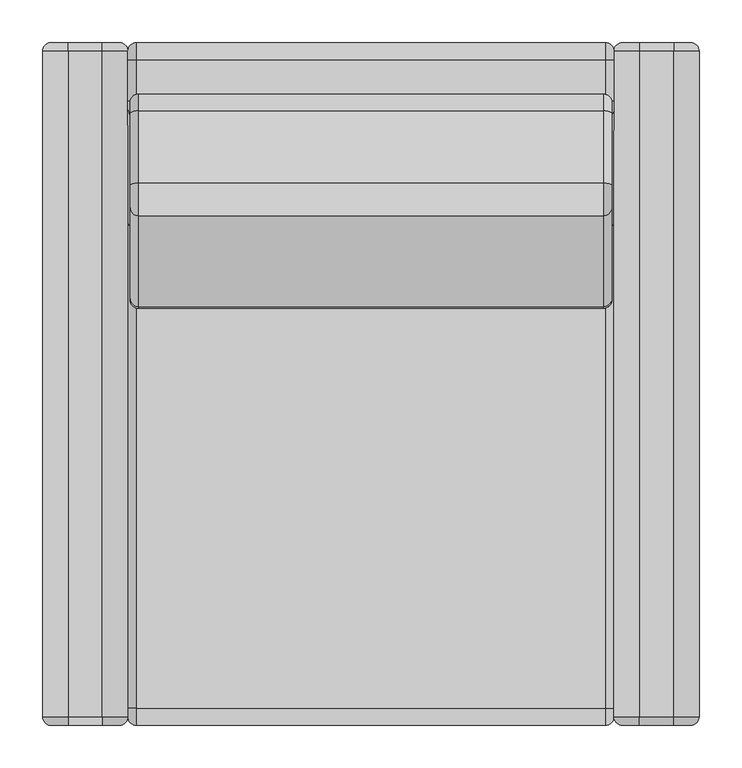
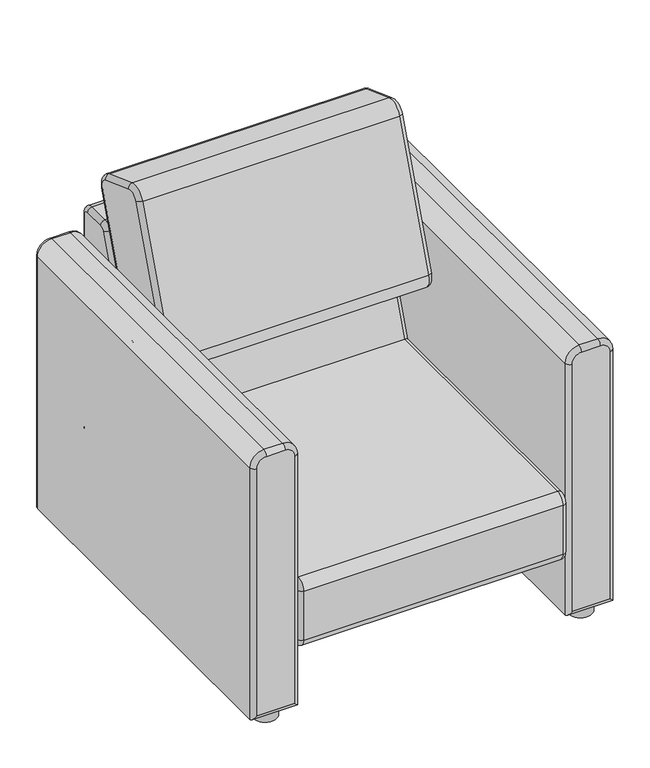
"""IFC4 building model written with IfcOpenShell, lengths in millimetres: furniture geometry."""

from ifc_helpers import new_model, si_unit, point, frame, frame_2d, origin, origin_with_axes, place, context, project, spatial, circle_curve, ellipse_curve, trimmed, segment, composite_curve, outline, extrude, source, transform, mapped, element, save
from ifc_brep_helpers import plane_surface, cylinder_surface, revolved_surface, advanced_brep


def furniture_f28dd14e(model_context):
    return source(origin(), model_context, "Body", "SolidModel", [
        advanced_brep(
        [(-375.0, 0.0, 590.0), (-375.0, 0.0, 35.0), (-295.0, 0.0, 35.0), (-295.0, 0.0, 590.0), (-315.0, 0.0, 610.0), (-355.0, 0.0, 610.0), (-295.0, 800.0, 590.0), (-295.0, 800.0, 35.0), (-375.0, 800.0, 35.0), (-375.0, 800.0, 590.0), (-355.0, 800.0, 610.0), (-315.0, 800.0, 610.0), (-285.0, 9.9999877, 590.0), (-285.0, 790.0000093, 590.0), (-315.0, 790.0, 620.0), (-315.0, 10.0, 620.0), (-355.0, 9.9999878, 620.0), (-355.0, 790.0, 620.0), (-385.0, 790.0, 590.0), (-385.0, 9.9999878, 590.0), (-285.0, 10.0, 25.0), (-285.0, 790.0, 25.0), (-385.0, 10.0, 25.0), (-385.0, 790.0, 25.0)],
        [
            (0, 1),
            (1, 2),
            (2, 3),
            (3, 4, circle_curve(frame((-315.0, 0.0, 590.0), z_axis=(0.0, -1.0, 0.0), x_axis=(0.0, 0.0, 1.0)), 20.0)),
            (4, 5),
            (5, 0, circle_curve(frame((-355.0, 0.0, 590.0), z_axis=(0.0, -1.0, 0.0), x_axis=(-1.0, 0.0, 0.0)), 20.0)),
            (6, 7),
            (7, 8),
            (8, 9),
            (9, 10, circle_curve(frame((-355.0, 800.0, 590.0), z_axis=(0.0, 1.0, 0.0), x_axis=(0.0, 0.0, 1.0)), 20.0)),
            (10, 11),
            (11, 6, circle_curve(frame((-315.0, 800.0, 590.0), z_axis=(0.0, 1.0, 0.0), x_axis=(1.0, 0.0, 0.0)), 20.0)),
            (12, 13),
            (13, 14, circle_curve(frame((-315.0, 790.0, 590.0), z_axis=(0.0, -1.0, 0.0), x_axis=(-1.0, 0.0, 0.0)), 30.0)),
            (14, 15),
            (15, 12, circle_curve(frame((-315.0, 10.0, 590.0), z_axis=(0.0, 1.0, 0.0), x_axis=(-1.0, 0.0, 0.0)), 30.0)),
            (16, 17),
            (17, 18, circle_curve(frame((-355.0, 790.0, 590.0), z_axis=(0.0, -1.0, 0.0), x_axis=(-1.0, 0.0, 0.0)), 30.0)),
            (18, 19),
            (19, 16, circle_curve(frame((-355.0, 10.0, 590.0), z_axis=(0.0, 1.0, 0.0), x_axis=(-1.0, 0.0, 0.0)), 30.0)),
            (20, 21),
            (21, 13),
            (12, 20),
            (22, 23),
            (23, 21),
            (20, 22),
            (18, 23),
            (22, 19),
            (14, 17),
            (16, 15),
            (19, 0, circle_curve(frame((-375.0, 10.0, 590.0), z_axis=(0.0, 0.0, 1.0), x_axis=(-1.0, 0.0, 0.0)), 10.0)),
            (5, 16, circle_curve(frame((-355.0, 10.0, 610.0), z_axis=(-1.0, 0.0, 0.0), x_axis=(0.0, 0.0, 1.0)), 10.0)),
            (4, 15, circle_curve(frame((-315.0, 10.0, 610.0), z_axis=(-1.0, 0.0, 0.0), x_axis=(0.0, 0.0, 1.0)), 10.0)),
            (3, 12, circle_curve(frame((-295.0, 10.0, 590.0), z_axis=(0.0, 0.0, 1.0), x_axis=(1.0, 0.0, 0.0)), 10.0)),
            (2, 20, ellipse_curve(frame((-295.0, 10.0, 35.0), z_axis=(0.7071067811865458, 0.0, 0.7071067811865492), x_axis=(0.7071067811865492, 0.0, -0.7071067811865458)), 14.1421356, 10.0)),
            (1, 22, ellipse_curve(frame((-375.0, 10.0, 35.0), z_axis=(0.7071067811865492, 0.0, -0.7071067811865457), x_axis=(-0.707106781186546, 0.0, -0.7071067811865491)), 14.1421356, 10.0)),
            (13, 6, circle_curve(frame((-295.0, 790.0, 590.0), z_axis=(0.0, 0.0, 1.0), x_axis=(-1.0, 0.0, 0.0)), 10.0)),
            (11, 14, circle_curve(frame((-315.0, 790.0, 610.0), z_axis=(1.0, 0.0, 0.0), x_axis=(0.0, 0.0, -1.0)), 10.0)),
            (10, 17, circle_curve(frame((-355.0, 790.0, 610.0), z_axis=(1.0, 0.0, 0.0), x_axis=(0.0, 0.0, -1.0)), 10.0)),
            (9, 18, circle_curve(frame((-375.0, 790.0, 590.0), z_axis=(0.0, 0.0, 1.0), x_axis=(1.0, 0.0, 0.0)), 10.0)),
            (8, 23, ellipse_curve(frame((-375.0, 790.0, 35.0), z_axis=(-0.7071067811865492, 0.0, 0.7071067811865458), x_axis=(-0.7071067811865457, 0.0, -0.7071067811865492)), 14.1421356, 10.0)),
            (7, 21, ellipse_curve(frame((-295.0, 790.0, 35.0), z_axis=(-0.707106781186546, 0.0, -0.7071067811865491), x_axis=(0.707106781186549, 0.0, -0.707106781186546)), 14.1421356, 10.0)),
        ],
        [
            plane_surface(frame((-345.0, 0.0, 590.0), z_axis=(0.0, -1.0, 0.0), x_axis=(0.0, 0.0, 1.0))),
            plane_surface(frame((-345.0, 800.0, 590.0), z_axis=(0.0, 1.0, 0.0), x_axis=(0.0, 0.0, -1.0))),
            cylinder_surface(frame((-315.0, 800.0, 590.0), z_axis=(0.0, -1.0, 0.0), x_axis=(-1.0, 0.0, 0.0)), 30.0),
            cylinder_surface(frame((-355.0, 800.0, 590.0), z_axis=(0.0, -1.0, 0.0), x_axis=(-1.0, 0.0, 0.0)), 30.0),
            plane_surface(frame((-285.0, 0.0, 590.0), z_axis=(1.0, 0.0, 0.0), x_axis=(0.0, 1.0, 0.0))),
            plane_surface(frame((-285.0, 0.0, 25.0), z_axis=(0.0, 0.0, -1.0), x_axis=(0.0, 1.0, 0.0))),
            plane_surface(frame((-385.0, 0.0, 25.0), z_axis=(-1.0, 0.0, 0.0), x_axis=(0.0, 1.0, 0.0))),
            plane_surface(frame((-355.0, 0.0, 620.0), z_axis=(0.0, 0.0, 1.0), x_axis=(0.0, 1.0, 0.0))),
            revolved_surface(trimmed(ellipse_curve(frame((-375.0, 10.0, 590.0), z_axis=(0.0, 0.0, 1.0), x_axis=(-1.0, 0.0, 0.0)), 10.0, 10.0), [point((-385.0, 10.0, 590.0))], [point((-375.0, 0.0, 590.0))], True, "CARTESIAN"), (-355.0, 0.0, 590.0), (0.0, -1.0, 0.0)),
            cylinder_surface(frame((-355.0, 10.0, 610.0), z_axis=(1.0, 0.0, 0.0), x_axis=(0.0, 0.0, 1.0)), 10.0),
            revolved_surface(trimmed(ellipse_curve(frame((-315.0, 10.0, 610.0), z_axis=(1.0, 0.0, 0.0), x_axis=(0.0, 0.0, 1.0)), 10.0, 10.0), [point((-315.0, 10.0, 620.0))], [point((-315.0, 0.0, 610.0))], True, "CARTESIAN"), (-315.0, 0.0, 590.0), (0.0, -1.0, 0.0)),
            cylinder_surface(frame((-295.0, 10.0, 590.0), z_axis=(0.0, 0.0, -1.0), x_axis=(1.0, 0.0, 0.0)), 10.0),
            cylinder_surface(frame((-285.0, 10.0, 35.0), z_axis=(-1.0, 0.0, 0.0), x_axis=(0.0, 0.0, -1.0)), 10.0),
            cylinder_surface(frame((-375.0, 10.0, 25.0), z_axis=(0.0, 0.0, 1.0), x_axis=(-1.0, 0.0, 0.0)), 10.0),
            revolved_surface(trimmed(ellipse_curve(frame((-295.0, 790.0, 590.0), z_axis=(0.0, 0.0, 1.0), x_axis=(-1.0, 0.0, 0.0)), 10.0, 10.0), [point((-285.0, 790.0, 590.0))], [point((-295.0, 800.0, 590.0))], True, "CARTESIAN"), (-315.0, 800.0, 590.0), (0.0, 1.0, 0.0)),
            cylinder_surface(frame((-315.0, 790.0, 610.0), z_axis=(-1.0, 0.0, 0.0), x_axis=(0.0, 0.0, -1.0)), 10.0),
            revolved_surface(trimmed(ellipse_curve(frame((-355.0, 790.0, 610.0), z_axis=(-1.0, 0.0, 0.0), x_axis=(0.0, 0.0, -1.0)), 10.0, 10.0), [point((-355.0, 790.0, 620.0))], [point((-355.0, 800.0, 610.0))], True, "CARTESIAN"), (-355.0, 800.0, 590.0), (0.0, 1.0, 0.0)),
            cylinder_surface(frame((-375.0, 790.0, 590.0), z_axis=(0.0, 0.0, -1.0), x_axis=(1.0, 0.0, 0.0)), 10.0),
            cylinder_surface(frame((-385.0, 790.0, 35.0), z_axis=(1.0, 0.0, 0.0), x_axis=(0.0, 0.0, 1.0)), 10.0),
            cylinder_surface(frame((-295.0, 790.0, 25.0), z_axis=(0.0, 0.0, 1.0), x_axis=(-1.0, 0.0, 0.0)), 10.0),
        ],
        [
            (0, [[1, 2, 3, 4, 5, 6]]),
            (1, [[7, 8, 9, 10, 11, 12]]),
            (2, [[13, 14, 15, 16]]),
            (3, [[17, 18, 19, 20]]),
            (4, [[21, 22, -13, 23]]),
            (5, [[24, 25, -21, 26]]),
            (6, [[-19, 27, -24, 28]]),
            (7, [[-15, 29, -17, 30]]),
            (8, [[-20, 31, -6, 32]]),
            (9, [[-5, 33, -30, -32]]),
            (10, [[-4, 34, -16, -33]]),
            (11, [[-3, 35, -23, -34]]),
            (12, [[-2, 36, -26, -35]]),
            (13, [[-28, -36, -1, -31]]),
            (14, [[-14, 37, -12, 38]]),
            (15, [[-11, 39, -29, -38]]),
            (16, [[-10, 40, -18, -39]]),
            (17, [[-9, 41, -27, -40]]),
            (18, [[-8, 42, -25, -41]]),
            (19, [[-22, -42, -7, -37]]),
        ],
    ),
        extrude(outline(composite_curve([segment(trimmed(circle_curve(frame_2d((-335.0, 760.0)), 25.0), [point((-310.0, 760.0))], [point((-360.0, 760.0))], False, "CARTESIAN"), True, "CONTINUOUS"), segment(trimmed(circle_curve(frame_2d((-335.0, 760.0)), 25.0), [point((-360.0, 760.0))], [point((-310.0, 760.0))], False, "CARTESIAN"), True, "CONTINUOUS")], self_intersect=False)), origin_with_axes(), (0.0, 0.0, 1.0), 25.0),
        extrude(outline(composite_curve([segment(trimmed(circle_curve(frame_2d((-335.0, 40.0)), 25.0), [point((-310.0, 40.0))], [point((-360.0, 40.0))], False, "CARTESIAN"), True, "CONTINUOUS"), segment(trimmed(circle_curve(frame_2d((-335.0, 40.0)), 25.0), [point((-360.0, 40.0))], [point((-310.0, 40.0))], False, "CARTESIAN"), True, "CONTINUOUS")], self_intersect=False)), origin_with_axes(), (0.0, 0.0, 1.0), 25.0),
        advanced_brep(
        [(375.0, 0.0, 590.0), (355.0, 0.0, 610.0), (315.0, 0.0, 610.0), (295.0, 0.0, 590.0), (295.0, 0.0, 35.0), (375.0, 0.0, 35.0), (295.0, 800.0, 590.0), (315.0, 800.0, 610.0), (355.0, 800.0, 610.0), (375.0, 800.0, 590.0), (375.0, 800.0, 35.0), (295.0, 800.0, 35.0), (285.0, 10.0, 590.0), (315.0, 10.0, 620.0), (315.0, 790.000012, 620.0), (285.0, 790.0, 590.0), (355.0, 10.0, 620.0), (385.0, 10.0, 590.0), (385.0, 790.0000092, 590.0), (355.0, 790.0, 620.0), (285.0, 10.0, 25.0), (285.0, 790.0, 25.0), (385.0, 10.0, 25.0), (385.0, 790.0, 25.0)],
        [
            (0, 1, circle_curve(frame((355.0, 0.0, 590.0), z_axis=(0.0, -1.0, 0.0), x_axis=(1.0, 0.0, 0.0)), 20.0)),
            (1, 2),
            (2, 3, circle_curve(frame((315.0, 0.0, 590.0), z_axis=(0.0, -1.0, 0.0), x_axis=(0.0, 0.0, 1.0)), 20.0)),
            (3, 4),
            (4, 5),
            (5, 0),
            (6, 7, circle_curve(frame((315.0, 800.0, 590.0), z_axis=(0.0, 1.0, 0.0), x_axis=(-1.0, 0.0, 0.0)), 20.0)),
            (7, 8),
            (8, 9, circle_curve(frame((355.0, 800.0, 590.0), z_axis=(0.0, 1.0, 0.0), x_axis=(0.0, 0.0, 1.0)), 20.0)),
            (9, 10),
            (10, 11),
            (11, 6),
            (12, 13, circle_curve(frame((315.0, 10.0, 590.0), z_axis=(0.0, 1.0, 0.0), x_axis=(1.0, 0.0, 0.0)), 30.0)),
            (13, 14),
            (14, 15, circle_curve(frame((315.0, 790.0, 590.0), z_axis=(0.0, -1.0, 0.0), x_axis=(1.0, 0.0, 0.0)), 30.0)),
            (15, 12),
            (16, 17, circle_curve(frame((355.0, 10.0, 590.0), z_axis=(0.0, 1.0, 0.0), x_axis=(1.0, 0.0, 0.0)), 30.0)),
            (17, 18),
            (18, 19, circle_curve(frame((355.0, 790.0, 590.0), z_axis=(0.0, -1.0, 0.0), x_axis=(1.0, 0.0, 0.0)), 30.0)),
            (19, 16),
            (20, 12),
            (15, 21),
            (21, 20),
            (22, 20),
            (21, 23),
            (23, 22),
            (17, 22),
            (23, 18),
            (13, 16),
            (19, 14),
            (16, 1, circle_curve(frame((355.0, 10.0, 610.0), z_axis=(1.0, 0.0, 0.0), x_axis=(0.0, 0.0, 1.0)), 10.0)),
            (0, 17, circle_curve(frame((375.0, 10.0, 590.0), z_axis=(0.0, 0.0, 1.0), x_axis=(1.0, 0.0, 0.0)), 10.0)),
            (13, 2, circle_curve(frame((315.0, 10.0, 610.0), z_axis=(1.0, 0.0, 0.0), x_axis=(0.0, 0.0, 1.0)), 10.0)),
            (12, 3, circle_curve(frame((295.0, 10.0, 590.0), z_axis=(0.0, 0.0, 1.0), x_axis=(-1.0, 0.0, 0.0)), 10.0)),
            (20, 4, ellipse_curve(frame((295.0, 10.0, 35.0), z_axis=(-0.7071067811865458, 0.0, 0.7071067811865492), x_axis=(-0.7071067811865492, 0.0, -0.7071067811865458)), 14.1421356, 10.0)),
            (22, 5, ellipse_curve(frame((375.0, 10.0, 35.0), z_axis=(-0.7071067811865492, 0.0, -0.7071067811865457), x_axis=(0.707106781186546, 0.0, -0.7071067811865491)), 14.1421356, 10.0)),
            (14, 7, circle_curve(frame((315.0, 790.0, 610.0), z_axis=(-1.0, 0.0, 0.0), x_axis=(0.0, 0.0, -1.0)), 10.0)),
            (6, 15, circle_curve(frame((295.0, 790.0, 590.0), z_axis=(0.0, 0.0, 1.0), x_axis=(1.0, 0.0, 0.0)), 10.0)),
            (19, 8, circle_curve(frame((355.0, 790.0, 610.0), z_axis=(-1.0, 0.0, 0.0), x_axis=(0.0, 0.0, -1.0)), 10.0)),
            (18, 9, circle_curve(frame((375.0, 790.0, 590.0), z_axis=(0.0, 0.0, 1.0), x_axis=(-1.0, 0.0, 0.0)), 10.0)),
            (23, 10, ellipse_curve(frame((375.0, 790.0, 35.0), z_axis=(0.7071067811865492, 0.0, 0.7071067811865458), x_axis=(0.7071067811865457, 0.0, -0.7071067811865492)), 14.1421356, 10.0)),
            (21, 11, ellipse_curve(frame((295.0, 790.0, 35.0), z_axis=(0.707106781186546, 0.0, -0.7071067811865491), x_axis=(-0.707106781186549, 0.0, -0.707106781186546)), 14.1421356, 10.0)),
        ],
        [
            plane_surface(frame((345.0, 0.0, 590.0), z_axis=(0.0, -1.0, 0.0), x_axis=(0.0, 0.0, 1.0))),
            plane_surface(frame((345.0, 800.0, 590.0), z_axis=(0.0, 1.0, 0.0), x_axis=(0.0, 0.0, -1.0))),
            cylinder_surface(frame((315.0, 800.0, 590.0), z_axis=(0.0, -1.0, 0.0), x_axis=(1.0, 0.0, 0.0)), 30.0),
            cylinder_surface(frame((355.0, 800.0, 590.0), z_axis=(0.0, -1.0, 0.0), x_axis=(1.0, 0.0, 0.0)), 30.0),
            plane_surface(frame((285.0, 0.0, 590.0), z_axis=(-1.0, 0.0, 0.0), x_axis=(0.0, 1.0, 0.0))),
            plane_surface(frame((285.0, 0.0, 25.0), z_axis=(0.0, 0.0, -1.0), x_axis=(0.0, 1.0, 0.0))),
            plane_surface(frame((385.0, 0.0, 25.0), z_axis=(1.0, 0.0, 0.0), x_axis=(0.0, 1.0, 0.0))),
            plane_surface(frame((355.0, 0.0, 620.0), z_axis=(0.0, 0.0, 1.0), x_axis=(0.0, 1.0, 0.0))),
            revolved_surface(trimmed(ellipse_curve(frame((375.0, 10.0, 590.0), z_axis=(0.0, 0.0, -1.0), x_axis=(1.0, 0.0, 0.0)), 10.0, 10.0), [point((385.0, 10.0, 590.0))], [point((375.0, 0.0, 590.0))], True, "CARTESIAN"), (355.0, 0.0, 590.0), (0.0, -1.0, 0.0)),
            cylinder_surface(frame((355.0, 10.0, 610.0), z_axis=(-1.0, 0.0, 0.0), x_axis=(0.0, 0.0, 1.0)), 10.0),
            revolved_surface(trimmed(ellipse_curve(frame((315.0, 10.0, 610.0), z_axis=(1.0, 0.0, 0.0), x_axis=(0.0, 0.0, 1.0)), 10.0, 10.0), [point((315.0, 10.0, 620.0))], [point((315.0, 0.0, 610.0))], True, "CARTESIAN"), (315.0, 0.0, 590.0), (0.0, -1.0, 0.0)),
            cylinder_surface(frame((295.0, 10.0, 590.0), z_axis=(0.0, 0.0, -1.0), x_axis=(-1.0, 0.0, 0.0)), 10.0),
            cylinder_surface(frame((285.0, 10.0, 35.0), z_axis=(1.0, 0.0, 0.0), x_axis=(0.0, 0.0, -1.0)), 10.0),
            cylinder_surface(frame((375.0, 10.0, 25.0), z_axis=(0.0, 0.0, 1.0), x_axis=(1.0, 0.0, 0.0)), 10.0),
            revolved_surface(trimmed(ellipse_curve(frame((295.0, 790.0, 590.0), z_axis=(0.0, 0.0, -1.0), x_axis=(1.0, 0.0, 0.0)), 10.0, 10.0), [point((285.0, 790.0, 590.0))], [point((295.0, 800.0, 590.0))], True, "CARTESIAN"), (315.0, 800.0, 590.0), (0.0, 1.0, 0.0)),
            cylinder_surface(frame((315.0, 790.0, 610.0), z_axis=(1.0, 0.0, 0.0), x_axis=(0.0, 0.0, -1.0)), 10.0),
            revolved_surface(trimmed(ellipse_curve(frame((355.0, 790.0, 610.0), z_axis=(-1.0, 0.0, 0.0), x_axis=(0.0, 0.0, -1.0)), 10.0, 10.0), [point((355.0, 790.0, 620.0))], [point((355.0, 800.0, 610.0))], True, "CARTESIAN"), (355.0, 800.0, 590.0), (0.0, 1.0, 0.0)),
            cylinder_surface(frame((375.0, 790.0, 590.0), z_axis=(0.0, 0.0, -1.0), x_axis=(-1.0, 0.0, 0.0)), 10.0),
            cylinder_surface(frame((385.0, 790.0, 35.0), z_axis=(-1.0, 0.0, 0.0), x_axis=(0.0, 0.0, 1.0)), 10.0),
            cylinder_surface(frame((295.0, 790.0, 25.0), z_axis=(0.0, 0.0, 1.0), x_axis=(1.0, 0.0, 0.0)), 10.0),
        ],
        [
            (0, [[1, 2, 3, 4, 5, 6]]),
            (1, [[7, 8, 9, 10, 11, 12]]),
            (2, [[13, 14, 15, 16]]),
            (3, [[17, 18, 19, 20]]),
            (4, [[21, -16, 22, 23]]),
            (5, [[24, -23, 25, 26]]),
            (6, [[27, -26, 28, -18]]),
            (7, [[29, -20, 30, -14]]),
            (8, [[31, -1, 32, -17]]),
            (9, [[-31, -29, 33, -2]]),
            (10, [[-33, -13, 34, -3]]),
            (11, [[-34, -21, 35, -4]]),
            (12, [[-35, -24, 36, -5]]),
            (13, [[-32, -6, -36, -27]]),
            (14, [[37, -7, 38, -15]]),
            (15, [[-37, -30, 39, -8]]),
            (16, [[-39, -19, 40, -9]]),
            (17, [[-40, -28, 41, -10]]),
            (18, [[-41, -25, 42, -11]]),
            (19, [[-38, -12, -42, -22]]),
        ],
    ),
        extrude(outline(composite_curve([segment(trimmed(circle_curve(frame_2d((335.0, 760.0)), 25.0), [point((310.0, 760.0))], [point((360.0, 760.0))], False, "CARTESIAN"), True, "CONTINUOUS"), segment(trimmed(circle_curve(frame_2d((335.0, 760.0)), 25.0), [point((360.0, 760.0))], [point((310.0, 760.0))], False, "CARTESIAN"), True, "CONTINUOUS")], self_intersect=False)), origin_with_axes(), (0.0, 0.0, 1.0), 25.0),
        extrude(outline(composite_curve([segment(trimmed(circle_curve(frame_2d((335.0, 40.0)), 25.0), [point((310.0, 40.0))], [point((360.0, 40.0))], False, "CARTESIAN"), True, "CONTINUOUS"), segment(trimmed(circle_curve(frame_2d((335.0, 40.0)), 25.0), [point((360.0, 40.0))], [point((310.0, 40.0))], False, "CARTESIAN"), True, "CONTINUOUS")], self_intersect=False)), origin_with_axes(), (0.0, 0.0, 1.0), 25.0),
        advanced_brep(
        [(285.0, 731.2835554, 660.0), (285.0, 721.8866292, 653.4202014), (285.0, 589.6124934, 290.0), (285.0, 20.0, 290.0), (285.0, 10.0, 280.0), (285.0, 10.0, 170.0), (285.0, 20.0, 160.0), (285.0, 780.0, 160.0), (285.0, 790.0, 170.0), (285.0, 790.0, 650.0), (285.0, 780.0, 660.0), (-285.0, 780.0, 660.0), (-285.0, 790.0, 650.0), (-285.0, 790.0, 170.0), (-285.0, 780.0, 160.0), (-285.0, 20.0, 160.0), (-285.0, 10.0, 170.0), (-285.0, 10.0, 280.0), (-285.0, 20.0, 290.0), (-285.0, 589.6124934, 290.0), (-285.0, 721.8866292, 653.4202014), (-285.0, 731.2835554, 660.0), (-275.0, 731.2835554, 670.0), (-275.0, 712.489703, 656.8404029), (275.0000092, 712.489703, 656.8404029), (275.0, 731.2835554, 670.0), (-275.0, 582.610418, 300.0), (275.0, 582.610418, 300.0), (-275.0, 20.0, 300.0), (275.0, 20.0, 300.0), (-275.0, 0.0, 280.0), (275.0000094, 0.0, 280.0), (-275.0, 0.0, 170.0), (275.0, 0.0, 170.0), (-275.0, 20.0, 150.0), (275.0000094, 20.0, 150.0), (-275.0, 780.0, 150.0), (275.0, 780.0, 150.0), (-275.0, 800.0, 170.0), (275.0000094, 800.0, 170.0), (-275.0, 800.0, 650.0), (275.0, 800.0, 650.0), (-275.0, 780.0, 670.0), (275.0000094, 780.0, 670.0)],
        [
            (0, 1, circle_curve(frame((285.0, 731.2835554, 650.0), z_axis=(1.0, 0.0, 0.0), x_axis=(0.0, 0.0, 1.0)), 10.0)),
            (1, 2),
            (2, 3),
            (3, 4, circle_curve(frame((285.0, 20.0, 280.0), z_axis=(1.0, 0.0, 0.0), x_axis=(0.0, 0.0, 1.0)), 10.0)),
            (4, 5),
            (5, 6, circle_curve(frame((285.0, 20.0, 170.0), z_axis=(1.0, 0.0, 0.0), x_axis=(0.0, -1.0, 0.0)), 10.0)),
            (6, 7),
            (7, 8, circle_curve(frame((285.0, 780.0, 170.0), z_axis=(1.0, 0.0, 0.0), x_axis=(0.0, 0.0, -1.0)), 10.0)),
            (8, 9),
            (9, 10, circle_curve(frame((285.0, 780.0, 650.0), z_axis=(1.0, 0.0, 0.0), x_axis=(0.0, 1.0, 0.0)), 10.0)),
            (10, 0),
            (11, 12, circle_curve(frame((-285.0, 780.0, 650.0), z_axis=(-1.0, 0.0, 0.0), x_axis=(0.0, 0.0, 1.0)), 10.0)),
            (12, 13),
            (13, 14, circle_curve(frame((-285.0, 780.0, 170.0), z_axis=(-1.0, 0.0, 0.0), x_axis=(0.0, 1.0, 0.0)), 10.0)),
            (14, 15),
            (15, 16, circle_curve(frame((-285.0, 20.0, 170.0), z_axis=(-1.0, 0.0, 0.0), x_axis=(0.0, 0.0, -1.0)), 10.0)),
            (16, 17),
            (17, 18, circle_curve(frame((-285.0, 20.0, 280.0), z_axis=(-1.0, 0.0, 0.0), x_axis=(0.0, -1.0, 0.0)), 10.0)),
            (18, 19),
            (19, 20),
            (20, 21, circle_curve(frame((-285.0, 731.2835554, 650.0), z_axis=(-1.0, 0.0, 0.0), x_axis=(0.0, -0.9396926207859061, 0.34202014332567493)), 10.0)),
            (21, 11),
            (22, 23, circle_curve(frame((-275.0, 731.2835554, 650.0), z_axis=(1.0, 0.0, 0.0), x_axis=(0.0, 1.0, 0.0)), 20.0)),
            (23, 24),
            (24, 25, circle_curve(frame((275.0, 731.2835554, 650.0), z_axis=(-1.0, 0.0, 0.0), x_axis=(0.0, 1.0, 0.0)), 20.0)),
            (25, 22),
            (23, 26),
            (26, 27),
            (27, 24),
            (26, 28),
            (28, 29),
            (29, 27),
            (28, 30, circle_curve(frame((-275.0, 20.0, 280.0), z_axis=(1.0, 0.0, 0.0), x_axis=(0.0, 1.0, 0.0)), 20.0)),
            (30, 31),
            (31, 29, circle_curve(frame((275.0, 20.0, 280.0), z_axis=(-1.0, 0.0, 0.0), x_axis=(0.0, 1.0, 0.0)), 20.0)),
            (30, 32),
            (32, 33),
            (33, 31),
            (32, 34, circle_curve(frame((-275.0, 20.0, 170.0), z_axis=(1.0, 0.0, 0.0), x_axis=(0.0, 1.0, 0.0)), 20.0)),
            (34, 35),
            (35, 33, circle_curve(frame((275.0, 20.0, 170.0), z_axis=(-1.0, 0.0, 0.0), x_axis=(0.0, 1.0, 0.0)), 20.0)),
            (34, 36),
            (36, 37),
            (37, 35),
            (36, 38, circle_curve(frame((-275.0, 780.0, 170.0), z_axis=(1.0, 0.0, 0.0), x_axis=(0.0, 1.0, 0.0)), 20.0)),
            (38, 39),
            (39, 37, circle_curve(frame((275.0, 780.0, 170.0), z_axis=(-1.0, 0.0, 0.0), x_axis=(0.0, 1.0, 0.0)), 20.0)),
            (38, 40),
            (40, 41),
            (41, 39),
            (40, 42, circle_curve(frame((-275.0, 780.0, 650.0), z_axis=(1.0, 0.0, 0.0), x_axis=(0.0, 1.0, 0.0)), 20.0)),
            (42, 43),
            (43, 41, circle_curve(frame((275.0, 780.0, 650.0), z_axis=(-1.0, 0.0, 0.0), x_axis=(0.0, 1.0, 0.0)), 20.0)),
            (42, 22),
            (25, 43),
            (40, 12, circle_curve(frame((-275.0, 790.0, 650.0), z_axis=(0.0, 0.0, 1.0), x_axis=(-1.0, 0.0, 0.0)), 10.0)),
            (11, 42, circle_curve(frame((-275.0, 780.0, 660.0), z_axis=(0.0, 1.0, 0.0), x_axis=(-1.0, 0.0, 0.0)), 10.0)),
            (38, 13, circle_curve(frame((-275.0, 790.0, 170.0), z_axis=(0.0, 0.0, 1.0), x_axis=(-1.0, 0.0, 0.0)), 10.0)),
            (36, 14, circle_curve(frame((-275.0, 780.0, 160.0), z_axis=(0.0, 1.0, 0.0), x_axis=(-1.0, 0.0, 0.0)), 10.0)),
            (34, 15, circle_curve(frame((-275.0, 20.0, 160.0), z_axis=(0.0, 1.0, 0.0), x_axis=(-1.0, 0.0, 0.0)), 10.0)),
            (32, 16, circle_curve(frame((-275.0, 10.0, 170.0), z_axis=(0.0, 0.0, -1.0), x_axis=(-1.0, 0.0, 0.0)), 10.0)),
            (30, 17, circle_curve(frame((-275.0, 10.0, 280.0), z_axis=(0.0, 0.0, -1.0), x_axis=(-1.0, 0.0, 0.0)), 10.0)),
            (28, 18, circle_curve(frame((-275.0, 20.0, 290.0), z_axis=(0.0, -1.0, 0.0), x_axis=(-1.0, 0.0, 0.0)), 10.0)),
            (26, 19, ellipse_curve(frame((-275.0, 589.6124934, 290.0), z_axis=(0.0, -0.8191520442889938, -0.573576436351043), x_axis=(0.0, 0.5735764363510434, -0.8191520442889937)), 12.2077459, 10.0)),
            (23, 20, circle_curve(frame((-275.0, 721.8866292, 653.4202014), z_axis=(0.0, -0.34202014332567243, -0.9396926207859071), x_axis=(-1.0, 0.0, 0.0)), 10.0)),
            (22, 21, circle_curve(frame((-275.0, 731.2835554, 660.0), z_axis=(0.0, -1.0, 0.0), x_axis=(-1.0, 0.0, 0.0)), 10.0)),
            (24, 1, circle_curve(frame((275.0, 721.8866292, 653.4202014), z_axis=(0.0, 0.3420201433256801, 0.9396926207859043), x_axis=(1.0, 0.0, 0.0)), 10.0)),
            (0, 25, circle_curve(frame((275.0, 731.2835554, 660.0), z_axis=(0.0, -1.0, 0.0), x_axis=(1.0, 0.0, 0.0)), 10.0)),
            (27, 2, ellipse_curve(frame((275.0, 589.6124934, 290.0), z_axis=(0.0, 0.8191520442889938, 0.573576436351043), x_axis=(0.0, 0.5735764363510429, -0.8191520442889941)), 12.2077459, 10.0)),
            (29, 3, circle_curve(frame((275.0, 20.0, 290.0), z_axis=(0.0, 1.0, 0.0), x_axis=(1.0, 0.0, 0.0)), 10.0)),
            (31, 4, circle_curve(frame((275.0, 10.0, 280.0), z_axis=(0.0, 0.0, 1.0), x_axis=(1.0, 0.0, 0.0)), 10.0)),
            (33, 5, circle_curve(frame((275.0, 10.0, 170.0), z_axis=(0.0, 0.0, 1.0), x_axis=(1.0, 0.0, 0.0)), 10.0)),
            (35, 6, circle_curve(frame((275.0, 20.0, 160.0), z_axis=(0.0, -1.0, 0.0), x_axis=(1.0, 0.0, 0.0)), 10.0)),
            (37, 7, circle_curve(frame((275.0, 780.0, 160.0), z_axis=(0.0, -1.0, 0.0), x_axis=(1.0, 0.0, 0.0)), 10.0)),
            (39, 8, circle_curve(frame((275.0, 790.0, 170.0), z_axis=(0.0, 0.0, -1.0), x_axis=(1.0, 0.0, 0.0)), 10.0)),
            (41, 9, circle_curve(frame((275.0, 790.0, 650.0), z_axis=(0.0, 0.0, -1.0), x_axis=(1.0, 0.0, 0.0)), 10.0)),
            (43, 10, circle_curve(frame((275.0, 780.0, 660.0), z_axis=(0.0, 1.0, 0.0), x_axis=(1.0, 0.0, 0.0)), 10.0)),
        ],
        [
            plane_surface(frame((285.0, 751.2835554, 650.0), z_axis=(1.0, 0.0, 0.0), x_axis=(0.0, 0.0, 1.0))),
            plane_surface(frame((-285.0, 751.2835554, 650.0), z_axis=(-1.0, 0.0, 0.0), x_axis=(0.0, 0.0, -1.0))),
            cylinder_surface(frame((-285.0, 731.2835554, 650.0), z_axis=(1.0, 0.0, 0.0), x_axis=(0.0, 1.0, 0.0)), 20.0),
            plane_surface(frame((285.0, 712.489703, 656.8404029), z_axis=(0.0, -0.9396926207859071, 0.3420201433256725), x_axis=(-1.0, 0.0, 0.0))),
            plane_surface(frame((285.0, 582.610418, 300.0), z_axis=(0.0, 0.0, 1.0), x_axis=(-1.0, 0.0, 0.0))),
            cylinder_surface(frame((-285.0, 20.0, 280.0), z_axis=(1.0, 0.0, 0.0), x_axis=(0.0, 1.0, 0.0)), 20.0),
            plane_surface(frame((285.0, 0.0, 280.0), z_axis=(0.0, -1.0, 0.0), x_axis=(-1.0, 0.0, 0.0))),
            cylinder_surface(frame((-285.0, 20.0, 170.0), z_axis=(1.0, 0.0, 0.0), x_axis=(0.0, 1.0, 0.0)), 20.0),
            plane_surface(frame((285.0, 20.0, 150.0), z_axis=(0.0, 0.0, -1.0), x_axis=(-1.0, 0.0, 0.0))),
            cylinder_surface(frame((-285.0, 780.0, 170.0), z_axis=(1.0, 0.0, 0.0), x_axis=(0.0, 1.0, 0.0)), 20.0),
            plane_surface(frame((285.0, 800.0, 170.0), z_axis=(0.0, 1.0, 0.0), x_axis=(-1.0, 0.0, 0.0))),
            cylinder_surface(frame((-285.0, 780.0, 650.0), z_axis=(1.0, 0.0, 0.0), x_axis=(0.0, 1.0, 0.0)), 20.0),
            plane_surface(frame((285.0, 780.0, 670.0), z_axis=(0.0, 0.0, 1.0), x_axis=(-1.0, 0.0, 0.0))),
            revolved_surface(trimmed(ellipse_curve(frame((-275.0, 780.0, 660.0), z_axis=(0.0, -1.0, 0.0), x_axis=(-1.0, 0.0, 0.0)), 10.0, 10.0), [point((-275.0, 780.0, 670.0))], [point((-285.0, 780.0, 660.0))], True, "CARTESIAN"), (-285.0, 780.0, 650.0), (-1.0, 0.0, 0.0)),
            cylinder_surface(frame((-275.0, 790.0, 650.0), z_axis=(0.0, 0.0, -1.0), x_axis=(-1.0, 0.0, 0.0)), 10.0),
            revolved_surface(trimmed(ellipse_curve(frame((-275.0, 790.0, 170.0), z_axis=(0.0, 0.0, 1.0), x_axis=(-1.0, 0.0, 0.0)), 10.0, 10.0), [point((-275.0, 800.0, 170.0))], [point((-285.0, 790.0, 170.0))], True, "CARTESIAN"), (-285.0, 780.0, 170.0), (-1.0, 0.0, 0.0)),
            cylinder_surface(frame((-275.0, 780.0, 160.0), z_axis=(0.0, -1.0, 0.0), x_axis=(-1.0, 0.0, 0.0)), 10.0),
            revolved_surface(trimmed(ellipse_curve(frame((-275.0, 20.0, 160.0), z_axis=(0.0, 1.0, 0.0), x_axis=(-1.0, 0.0, 0.0)), 10.0, 10.0), [point((-275.0, 20.0, 150.0))], [point((-285.0, 20.0, 160.0))], True, "CARTESIAN"), (-285.0, 20.0, 170.0), (-1.0, 0.0, 0.0)),
            cylinder_surface(frame((-275.0, 10.0, 170.0), z_axis=(0.0, 0.0, 1.0), x_axis=(-1.0, 0.0, 0.0)), 10.0),
            revolved_surface(trimmed(ellipse_curve(frame((-275.0, 10.0, 280.0), z_axis=(0.0, 0.0, -1.0), x_axis=(-1.0, 0.0, 0.0)), 10.0, 10.0), [point((-275.0, 0.0, 280.0))], [point((-285.0, 10.0, 280.0))], True, "CARTESIAN"), (-285.0, 20.0, 280.0), (-1.0, 0.0, 0.0)),
            cylinder_surface(frame((-275.0, 20.0, 290.0), z_axis=(0.0, 1.0, 0.0), x_axis=(-1.0, 0.0, 0.0)), 10.0),
            cylinder_surface(frame((-275.0, 592.0073442, 296.5797986), z_axis=(0.0, 0.34202014332567243, 0.9396926207859071), x_axis=(-1.0, 0.0, 0.0)), 10.0),
            revolved_surface(trimmed(ellipse_curve(frame((-275.0, 721.8866292, 653.4202014), z_axis=(0.0, -0.3420201433256749, -0.9396926207859061), x_axis=(-1.0, 0.0, 0.0)), 10.0, 10.0), [point((-275.0, 712.489703, 656.8404029))], [point((-285.0, 721.8866292, 653.4202014))], True, "CARTESIAN"), (-285.0, 731.2835554, 650.0), (-1.0, 0.0, 0.0)),
            cylinder_surface(frame((-275.0, 731.2835554, 660.0), z_axis=(0.0, 1.0, 0.0), x_axis=(-1.0, 0.0, 0.0)), 10.0),
            revolved_surface(trimmed(ellipse_curve(frame((275.0, 731.2835554, 660.0), z_axis=(0.0, 1.0, 0.0), x_axis=(1.0, 0.0, 0.0)), 10.0, 10.0), [point((275.0, 731.2835554, 670.0))], [point((285.0, 731.2835554, 660.0))], True, "CARTESIAN"), (285.0, 731.2835554, 650.0), (1.0, 0.0, 0.0)),
            cylinder_surface(frame((275.0, 721.8866292, 653.4202014), z_axis=(0.0, -0.34202014332567254, -0.939692620785907), x_axis=(1.0, 0.0, 0.0)), 10.0),
            cylinder_surface(frame((275.0, 582.610418, 290.0), z_axis=(0.0, -1.0, 0.0), x_axis=(1.0, 0.0, 0.0)), 10.0),
            revolved_surface(trimmed(ellipse_curve(frame((275.0, 20.0, 290.0), z_axis=(0.0, 1.0, 0.0), x_axis=(1.0, 0.0, 0.0)), 10.0, 10.0), [point((275.0, 20.0, 300.0))], [point((285.0, 20.0, 290.0))], True, "CARTESIAN"), (285.0, 20.0, 280.0), (1.0, 0.0, 0.0)),
            cylinder_surface(frame((275.0, 10.0, 280.0), z_axis=(0.0, 0.0, -1.0), x_axis=(1.0, 0.0, 0.0)), 10.0),
            revolved_surface(trimmed(ellipse_curve(frame((275.0, 10.0, 170.0), z_axis=(0.0, 0.0, 1.0), x_axis=(1.0, 0.0, 0.0)), 10.0, 10.0), [point((275.0, 0.0, 170.0))], [point((285.0, 10.0, 170.0))], True, "CARTESIAN"), (285.0, 20.0, 170.0), (1.0, 0.0, 0.0)),
            cylinder_surface(frame((275.0, 20.0, 160.0), z_axis=(0.0, 1.0, 0.0), x_axis=(1.0, 0.0, 0.0)), 10.0),
            revolved_surface(trimmed(ellipse_curve(frame((275.0, 780.0, 160.0), z_axis=(0.0, -1.0, 0.0), x_axis=(1.0, 0.0, 0.0)), 10.0, 10.0), [point((275.0, 780.0, 150.0))], [point((285.0, 780.0, 160.0))], True, "CARTESIAN"), (285.0, 780.0, 170.0), (1.0, 0.0, 0.0)),
            cylinder_surface(frame((275.0, 790.0, 170.0), z_axis=(0.0, 0.0, 1.0), x_axis=(1.0, 0.0, 0.0)), 10.0),
            revolved_surface(trimmed(ellipse_curve(frame((275.0, 790.0, 650.0), z_axis=(0.0, 0.0, -1.0), x_axis=(1.0, 0.0, 0.0)), 10.0, 10.0), [point((275.0, 800.0, 650.0))], [point((285.0, 790.0, 650.0))], True, "CARTESIAN"), (285.0, 780.0, 650.0), (1.0, 0.0, 0.0)),
            cylinder_surface(frame((275.0, 780.0, 660.0), z_axis=(0.0, -1.0, 0.0), x_axis=(1.0, 0.0, 0.0)), 10.0),
        ],
        [
            (0, [[1, 2, 3, 4, 5, 6, 7, 8, 9, 10, 11]]),
            (1, [[12, 13, 14, 15, 16, 17, 18, 19, 20, 21, 22]]),
            (2, [[23, 24, 25, 26]]),
            (3, [[27, 28, 29, -24]]),
            (4, [[30, 31, 32, -28]]),
            (5, [[33, 34, 35, -31]]),
            (6, [[36, 37, 38, -34]]),
            (7, [[39, 40, 41, -37]]),
            (8, [[42, 43, 44, -40]]),
            (9, [[45, 46, 47, -43]]),
            (10, [[48, 49, 50, -46]]),
            (11, [[51, 52, 53, -49]]),
            (12, [[54, -26, 55, -52]]),
            (13, [[56, -12, 57, -51]]),
            (14, [[-56, -48, 58, -13]]),
            (15, [[-58, -45, 59, -14]]),
            (16, [[-59, -42, 60, -15]]),
            (17, [[-60, -39, 61, -16]]),
            (18, [[-61, -36, 62, -17]]),
            (19, [[-62, -33, 63, -18]]),
            (20, [[-63, -30, 64, -19]]),
            (21, [[-64, -27, 65, -20]]),
            (22, [[-65, -23, 66, -21]]),
            (23, [[-57, -22, -66, -54]]),
            (24, [[67, -1, 68, -25]]),
            (25, [[-67, -29, 69, -2]]),
            (26, [[-69, -32, 70, -3]]),
            (27, [[-70, -35, 71, -4]]),
            (28, [[-71, -38, 72, -5]]),
            (29, [[-72, -41, 73, -6]]),
            (30, [[-73, -44, 74, -7]]),
            (31, [[-74, -47, 75, -8]]),
            (32, [[-75, -50, 76, -9]]),
            (33, [[-76, -53, 77, -10]]),
            (34, [[-68, -11, -77, -55]]),
        ],
    ),
        advanced_brep(
        [(282.5, 499.8874666, 496.8626858), (282.5, 518.742541, 469.9348489), (282.5, 614.5185405, 469.9348489), (282.5, 633.3736149, 483.1373142), (282.5, 728.5847628, 744.7277933), (282.5, 716.5923743, 770.4455535), (282.5, 632.0200384, 801.2273664), (282.5, 606.3022782, 789.2349779), (-282.5, 518.742541, 469.9348489), (-282.5, 499.8874666, 496.8626858), (-282.5, 606.3022782, 789.2349779), (-282.5, 632.0200384, 801.2273664), (-282.5, 716.5923743, 770.4455535), (-282.5, 728.5847628, 744.7277933), (-282.5, 633.3736149, 483.1373142), (-282.5, 614.5185405, 469.9348489), (-272.5, 635.4402399, 810.6242926), (-272.5, 596.905352, 792.6551793), (272.5, 596.905352, 792.6551793), (272.5, 635.4402399, 810.6242926), (-272.5, 490.4905403, 500.2828873), (272.5, 490.4905403, 500.2828873), (-272.5, 518.742541, 459.9348489), (272.5, 518.742541, 459.9348489), (-272.5, 614.5185405, 459.9348489), (272.5, 614.5185405, 459.9348489), (-272.5, 642.7705411, 479.7171127), (272.5, 642.7705411, 479.7171127), (-272.5, 737.9816891, 741.3075918), (272.5, 737.9816891, 741.3075918), (-272.5, 720.0125757, 779.8424797), (272.5, 720.0125757, 779.8424797)],
        [
            (0, 1, circle_curve(frame((282.5, 518.742541, 490.0), z_axis=(1.0, 0.0, 0.0), x_axis=(0.0, 0.0, -1.0)), 20.0651511)),
            (1, 2),
            (2, 3, circle_curve(frame((282.5, 614.5185405, 490.0), z_axis=(1.0, 0.0, 0.0), x_axis=(0.0, 0.9396926207859085, -0.3420201433256683)), 20.0651511)),
            (3, 4),
            (4, 5, circle_curve(frame((282.5, 709.7296884, 751.5904791), z_axis=(1.0, 0.0, 0.0), x_axis=(0.0, 0.34202014332567177, 0.9396926207859073)), 20.0651511)),
            (5, 6),
            (6, 7, circle_curve(frame((282.5, 625.1573526, 782.372292), z_axis=(1.0, 0.0, 0.0), x_axis=(0.0, -0.9396926207859104, 0.3420201433256632)), 20.0651511)),
            (7, 0),
            (8, 9, circle_curve(frame((-282.5, 518.742541, 490.0), z_axis=(-1.0, 0.0, 0.0), x_axis=(0.0, 0.0, -1.0)), 20.0651511)),
            (9, 10),
            (10, 11, circle_curve(frame((-282.5, 625.1573526, 782.372292), z_axis=(-1.0, 0.0, 0.0), x_axis=(0.0, -0.9396926207859104, 0.3420201433256632)), 20.0651511)),
            (11, 12),
            (12, 13, circle_curve(frame((-282.5, 709.7296884, 751.5904791), z_axis=(-1.0, 0.0, 0.0), x_axis=(0.0, 0.34202014332567177, 0.9396926207859073)), 20.0651511)),
            (13, 14),
            (14, 15, circle_curve(frame((-282.5, 614.5185405, 490.0), z_axis=(-1.0, 0.0, 0.0), x_axis=(0.0, 0.9396926207859085, -0.3420201433256683)), 20.0651511)),
            (15, 8),
            (16, 17, circle_curve(frame((-272.5, 625.1573526, 782.372292), z_axis=(1.0, 0.0, 0.0), x_axis=(0.0, 1.0, 0.0)), 30.0651511)),
            (17, 18),
            (18, 19, circle_curve(frame((272.5, 625.1573526, 782.372292), z_axis=(-1.0, 0.0, 0.0), x_axis=(0.0, 1.0, 0.0)), 30.0651511)),
            (19, 16),
            (17, 20),
            (20, 21),
            (21, 18),
            (20, 22, circle_curve(frame((-272.5, 518.742541, 490.0), z_axis=(1.0, 0.0, 0.0), x_axis=(0.0, 1.0, 0.0)), 30.0651511)),
            (22, 23),
            (23, 21, circle_curve(frame((272.5, 518.742541, 490.0), z_axis=(-1.0, 0.0, 0.0), x_axis=(0.0, 1.0, 0.0)), 30.0651511)),
            (22, 24),
            (24, 25),
            (25, 23),
            (24, 26, circle_curve(frame((-272.5, 614.5185405, 490.0), z_axis=(1.0, 0.0, 0.0), x_axis=(0.0, 1.0, 0.0)), 30.0651511)),
            (26, 27),
            (27, 25, circle_curve(frame((272.5, 614.5185405, 490.0), z_axis=(-1.0, 0.0, 0.0), x_axis=(0.0, 1.0, 0.0)), 30.0651511)),
            (26, 28),
            (28, 29),
            (29, 27),
            (28, 30, circle_curve(frame((-272.5, 709.7296884, 751.5904791), z_axis=(1.0, 0.0, 0.0), x_axis=(0.0, 1.0, 0.0)), 30.0651511)),
            (30, 31),
            (31, 29, circle_curve(frame((272.5, 709.7296884, 751.5904791), z_axis=(-1.0, 0.0, 0.0), x_axis=(0.0, 1.0, 0.0)), 30.0651511)),
            (30, 16),
            (19, 31),
            (20, 9, circle_curve(frame((-272.5, 499.8874666, 496.8626858), z_axis=(0.0, -0.34202014332566166, -0.939692620785911), x_axis=(-1.0, 0.0, 0.0)), 10.0)),
            (8, 22, circle_curve(frame((-272.5, 518.742541, 469.9348489), z_axis=(0.0, -1.0, 0.0), x_axis=(-1.0, 0.0, 0.0)), 10.0)),
            (17, 10, circle_curve(frame((-272.5, 606.3022782, 789.2349779), z_axis=(0.0, -0.34202014332565833, -0.9396926207859122), x_axis=(-1.0, 0.0, 0.0)), 10.0)),
            (16, 11, circle_curve(frame((-272.5, 632.0200384, 801.2273664), z_axis=(0.0, -0.9396926207859083, 0.34202014332566916), x_axis=(-1.0, 0.0, 0.0)), 10.0)),
            (30, 12, circle_curve(frame((-272.5, 716.5923743, 770.4455535), z_axis=(0.0, -0.9396926207859225, 0.3420201433256301), x_axis=(-1.0, 0.0, 0.0)), 10.0)),
            (28, 13, circle_curve(frame((-272.5, 728.5847628, 744.7277933), z_axis=(0.0, 0.3420201433256681, 0.9396926207859086), x_axis=(-1.0, 0.0, 0.0)), 10.0)),
            (26, 14, circle_curve(frame((-272.5, 633.3736149, 483.1373142), z_axis=(0.0, 0.34202014332565617, 0.939692620785913), x_axis=(-1.0, 0.0, 0.0)), 10.0)),
            (24, 15, circle_curve(frame((-272.5, 614.5185405, 469.9348489), z_axis=(0.0, 0.9999999999999999, 0.0), x_axis=(-1.0, 0.0, 0.0)), 10.0)),
            (0, 21, circle_curve(frame((272.5, 499.8874666, 496.8626858), z_axis=(0.0, -0.34202014332566655, -0.9396926207859091), x_axis=(-1.0, 0.0, 0.0)), 10.0)),
            (23, 1, circle_curve(frame((272.5, 518.742541, 469.9348489), z_axis=(0.0, -1.0, 0.0), x_axis=(-1.0, 0.0, 0.0)), 10.0)),
            (7, 18, circle_curve(frame((272.5, 606.3022782, 789.2349779), z_axis=(0.0, -0.3420201433256584, -0.9396926207859122), x_axis=(-1.0, 0.0, 0.0)), 10.0)),
            (6, 19, circle_curve(frame((272.5, 632.0200384, 801.2273664), z_axis=(0.0, -0.9396926207859042, 0.3420201433256802), x_axis=(-1.0, 0.0, 0.0)), 10.0)),
            (5, 31, circle_curve(frame((272.5, 716.5923743, 770.4455535), z_axis=(0.0, -0.9396926207859225, 0.3420201433256302), x_axis=(-1.0, 0.0, 0.0)), 10.0)),
            (4, 29, circle_curve(frame((272.5, 728.5847628, 744.7277933), z_axis=(0.0, 0.3420201433256699, 0.939692620785908), x_axis=(-1.0, 0.0, 0.0)), 10.0)),
            (3, 27, circle_curve(frame((272.5, 633.3736149, 483.1373142), z_axis=(0.0, 0.3420201433256563, 0.9396926207859129), x_axis=(-1.0, 0.0, 0.0)), 10.0)),
            (2, 25, circle_curve(frame((272.5, 614.5185405, 469.9348489), z_axis=(0.0, 1.0, 0.0), x_axis=(-1.0, 0.0, 0.0)), 10.0)),
        ],
        [
            plane_surface(frame((282.5, 655.2225036, 782.372292), z_axis=(1.0, 0.0, 0.0), x_axis=(0.0, 0.0, 1.0))),
            plane_surface(frame((-282.5, 655.2225036, 782.372292), z_axis=(-1.0, 0.0, 0.0), x_axis=(0.0, 0.0, -1.0))),
            cylinder_surface(frame((-282.5, 625.1573526, 782.372292), z_axis=(1.0, 0.0, 0.0), x_axis=(0.0, 1.0, 0.0)), 30.0651511),
            plane_surface(frame((282.5, 596.905352, 792.6551793), z_axis=(0.0, -0.9396926207859123, 0.3420201433256582), x_axis=(-1.0, 0.0, 0.0))),
            cylinder_surface(frame((-282.5, 518.742541, 490.0), z_axis=(1.0, 0.0, 0.0), x_axis=(0.0, 1.0, 0.0)), 30.0651511),
            plane_surface(frame((282.5, 518.742541, 459.9348489), z_axis=(0.0, 0.0, -1.0), x_axis=(-1.0, 0.0, 0.0))),
            cylinder_surface(frame((-282.5, 614.5185405, 490.0), z_axis=(1.0, 0.0, 0.0), x_axis=(0.0, 1.0, 0.0)), 30.0651511),
            plane_surface(frame((282.5, 642.7705411, 479.7171127), z_axis=(0.0, 0.9396926207859131, -0.3420201433256561), x_axis=(-1.0, 0.0, 0.0))),
            cylinder_surface(frame((-282.5, 709.7296884, 751.5904791), z_axis=(1.0, 0.0, 0.0), x_axis=(0.0, 1.0, 0.0)), 30.0651511),
            plane_surface(frame((282.5, 720.0125757, 779.8424797), z_axis=(0.0, 0.34202014332562986, 0.9396926207859226), x_axis=(-1.0, 0.0, 0.0))),
            revolved_surface(trimmed(ellipse_curve(frame((-272.5, 518.742541, 469.9348489), z_axis=(0.0, 1.0, 0.0), x_axis=(-1.0, 0.0, 0.0)), 10.0, 10.0), [point((-272.5, 518.742541, 459.9348489))], [point((-282.5, 518.742541, 469.9348489))], True, "CARTESIAN"), (-282.5, 518.742541, 490.0), (-1.0, 0.0, 0.0)),
            cylinder_surface(frame((-272.5, 499.8874666, 496.8626858), z_axis=(0.0, 0.34202014332565833, 0.9396926207859122), x_axis=(-1.0, 0.0, 0.0)), 10.0),
            revolved_surface(trimmed(ellipse_curve(frame((-272.5, 606.3022782, 789.2349779), z_axis=(0.0, -0.3420201433256636, -0.9396926207859103), x_axis=(-1.0, 0.0, 0.0)), 10.0, 10.0), [point((-272.5, 596.905352, 792.6551793))], [point((-282.5, 606.3022782, 789.2349779))], True, "CARTESIAN"), (-282.5, 625.1573526, 782.372292), (-1.0, 0.0, 0.0)),
            cylinder_surface(frame((-272.5, 632.0200384, 801.2273664), z_axis=(0.0, 0.9396926207859225, -0.3420201433256301), x_axis=(-1.0, 0.0, 0.0)), 10.0),
            revolved_surface(trimmed(ellipse_curve(frame((-272.5, 716.5923743, 770.4455535), z_axis=(0.0, -0.9396926207859072, 0.34202014332567193), x_axis=(-1.0, 0.0, 0.0)), 10.0, 10.0), [point((-272.5, 720.0125757, 779.8424797))], [point((-282.5, 716.5923743, 770.4455535))], True, "CARTESIAN"), (-282.5, 709.7296884, 751.5904791), (-1.0, 0.0, 0.0)),
            cylinder_surface(frame((-272.5, 728.5847628, 744.7277933), z_axis=(0.0, -0.34202014332565617, -0.939692620785913), x_axis=(-1.0, 0.0, 0.0)), 10.0),
            revolved_surface(trimmed(ellipse_curve(frame((-272.5, 633.3736149, 483.1373142), z_axis=(0.0, 0.34202014332566844, 0.9396926207859085), x_axis=(-1.0, 0.0, 0.0)), 10.0, 10.0), [point((-272.5, 642.7705411, 479.7171127))], [point((-282.5, 633.3736149, 483.1373142))], True, "CARTESIAN"), (-282.5, 614.5185405, 490.0), (-1.0, 0.0, 0.0)),
            cylinder_surface(frame((-272.5, 614.5185405, 469.9348489), z_axis=(0.0, -1.0, 0.0), x_axis=(-1.0, 0.0, 0.0)), 10.0),
            revolved_surface(trimmed(ellipse_curve(frame((272.5, 518.742541, 469.9348489), z_axis=(0.0, 1.0, 0.0), x_axis=(-1.0, 0.0, 0.0)), 10.0, 10.0), [point((282.5, 518.742541, 469.9348489))], [point((272.5, 518.742541, 459.9348489))], True, "CARTESIAN"), (282.5, 518.742541, 490.0), (-1.0, 0.0, 0.0)),
            cylinder_surface(frame((272.5, 499.8874666, 496.8626858), z_axis=(0.0, 0.3420201433256584, 0.9396926207859122), x_axis=(-1.0, 0.0, 0.0)), 10.0),
            revolved_surface(trimmed(ellipse_curve(frame((272.5, 606.3022782, 789.2349779), z_axis=(0.0, -0.3420201433256636, -0.9396926207859103), x_axis=(-1.0, 0.0, 0.0)), 10.0, 10.0), [point((282.5, 606.3022782, 789.2349779))], [point((272.5, 596.905352, 792.6551793))], True, "CARTESIAN"), (282.5, 625.1573526, 782.372292), (-1.0, 0.0, 0.0)),
            cylinder_surface(frame((272.5, 632.0200384, 801.2273664), z_axis=(0.0, 0.9396926207859225, -0.3420201433256302), x_axis=(-1.0, 0.0, 0.0)), 10.0),
            revolved_surface(trimmed(ellipse_curve(frame((272.5, 716.5923743, 770.4455535), z_axis=(0.0, -0.9396926207859072, 0.34202014332567204), x_axis=(-1.0, 0.0, 0.0)), 10.0, 10.0), [point((282.5, 716.5923743, 770.4455535))], [point((272.5, 720.0125757, 779.8424797))], True, "CARTESIAN"), (282.5, 709.7296884, 751.5904791), (-1.0, 0.0, 0.0)),
            cylinder_surface(frame((272.5, 728.5847628, 744.7277933), z_axis=(0.0, -0.3420201433256563, -0.9396926207859129), x_axis=(-1.0, 0.0, 0.0)), 10.0),
            revolved_surface(trimmed(ellipse_curve(frame((272.5, 633.3736149, 483.1373142), z_axis=(0.0, 0.34202014332566855, 0.9396926207859084), x_axis=(-1.0, 0.0, 0.0)), 10.0, 10.0), [point((282.5, 633.3736149, 483.1373142))], [point((272.5, 642.7705411, 479.7171127))], True, "CARTESIAN"), (282.5, 614.5185405, 490.0), (-1.0, 0.0, 0.0)),
            cylinder_surface(frame((272.5, 614.5185405, 469.9348489), z_axis=(0.0, -1.0, 0.0), x_axis=(-1.0, 0.0, 0.0)), 10.0),
        ],
        [
            (0, [[1, 2, 3, 4, 5, 6, 7, 8]]),
            (1, [[9, 10, 11, 12, 13, 14, 15, 16]]),
            (2, [[17, 18, 19, 20]]),
            (3, [[21, 22, 23, -18]]),
            (4, [[24, 25, 26, -22]]),
            (5, [[27, 28, 29, -25]]),
            (6, [[30, 31, 32, -28]]),
            (7, [[33, 34, 35, -31]]),
            (8, [[36, 37, 38, -34]]),
            (9, [[39, -20, 40, -37]]),
            (10, [[41, -9, 42, -24]]),
            (11, [[-41, -21, 43, -10]]),
            (12, [[-43, -17, 44, -11]]),
            (13, [[-44, -39, 45, -12]]),
            (14, [[-45, -36, 46, -13]]),
            (15, [[-46, -33, 47, -14]]),
            (16, [[-47, -30, 48, -15]]),
            (17, [[-42, -16, -48, -27]]),
            (18, [[49, -26, 50, -1]]),
            (19, [[-49, -8, 51, -23]]),
            (20, [[-51, -7, 52, -19]]),
            (21, [[-52, -6, 53, -40]]),
            (22, [[-53, -5, 54, -38]]),
            (23, [[-54, -4, 55, -35]]),
            (24, [[-55, -3, 56, -32]]),
            (25, [[-50, -29, -56, -2]]),
        ],
    ),
    ])


if __name__ == "__main__":
    model = new_model("IFC4")
    model_context = context("Model", 3, world=origin())
    ifc_project = project(units=[si_unit("LENGTHUNIT", "METRE", prefix="MILLI")], contexts=[model_context])
    site = spatial("IfcSite", under=ifc_project)
    building = spatial("IfcBuilding", under=site)
    placement = place(None, origin())
    furniture_shape = furniture_f28dd14e(model_context)
    element("IfcFurniture", 1, at=placement, inside=building, context=model_context, shape_type="MappedRepresentation", body=[
        mapped(furniture_shape, transform((0.0, 0.0, 0.0), x_axis=(1.0, 0.0, 0.0), y_axis=(0.0, 1.0, 0.0), z_axis=(0.0, 0.0, 1.0))),
    ])
    save(model, "model.ifc")

# Revit data of these elements
# Type
#   Width [instance] = 2' - 6.31496"
#   Default Elevation = 0
